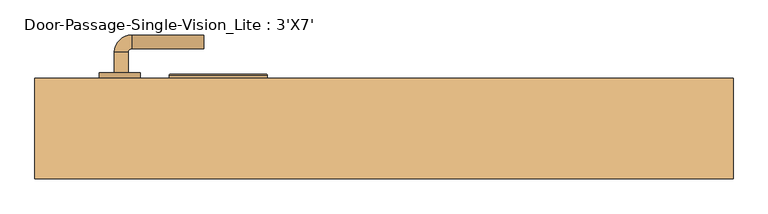
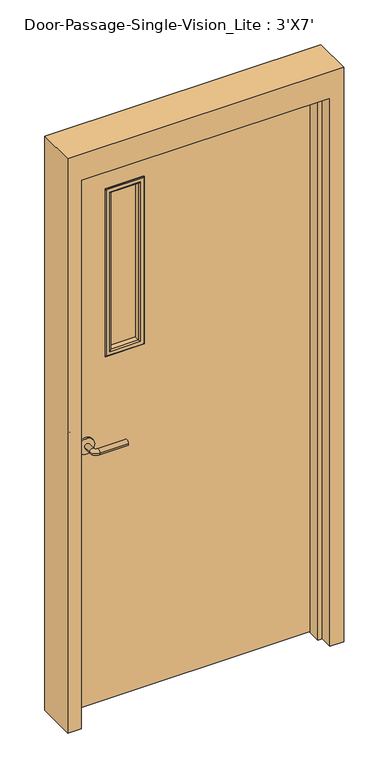
"""IFC4 building model written with IfcOpenShell, lengths in millimetres: door geometry, Door-Passage-Single-Vision_Lite : 3'X7'."""

from ifc_helpers import new_model, si_unit, point, frame, frame_2d, origin, place, context, project, spatial, polyline, circle_curve, ellipse_curve, trimmed, segment, composite_curve, outline, extrude, faceted_brep, source, transform, mapped, element, save
from ifc_brep_helpers import plane_surface, cylinder_surface, revolved_surface, advanced_brep


def door_passage_single_vision_lite_3_x7_440dd290(model_context):
    return source(origin(), model_context, "Body", "SolidModel", [
        advanced_brep(
        [(-392.190625, -14.35, 1016.0), (-372.190625, -14.35, 1016.0), (-372.190625, -44.35, 1016.0), (-392.190625, -44.35, 1016.0), (-367.190625, -49.35, 1016.0), (-367.190625, -69.35, 1016.0), (-262.190625, -69.35, 1016.0), (-262.190625, -49.35, 1016.0)],
        [
            (0, 1, circle_curve(frame((-382.190625, -14.35, 1016.0), z_axis=(0.0, 1.0, 0.0), x_axis=(1.0, 0.0, 0.0)), 10.0)),
            (1, 0, circle_curve(frame((-382.190625, -14.35, 1016.0), z_axis=(0.0, 1.0, 0.0), x_axis=(1.0, 0.0, 0.0)), 10.0)),
            (1, 2),
            (2, 3, circle_curve(frame((-382.190625, -44.35, 1016.0), z_axis=(0.0, 1.0, 0.0), x_axis=(1.0, 0.0, 0.0)), 10.0)),
            (3, 0),
            (3, 2, circle_curve(frame((-382.190625, -44.35, 1016.0), z_axis=(0.0, 1.0, 0.0), x_axis=(1.0, 0.0, 0.0)), 10.0)),
            (4, 5, circle_curve(frame((-367.190625, -59.35, 1016.0), z_axis=(-1.0, 0.0, 0.0), x_axis=(0.0, 1.0, 0.0)), 10.0)),
            (5, 3, circle_curve(frame((-367.190625, -44.35, 1016.0), z_axis=(0.0, 0.0, -1.0), x_axis=(-1.0, 0.0, 0.0)), 25.0)),
            (2, 4, circle_curve(frame((-367.190625, -44.35, 1016.0), z_axis=(0.0, 0.0, 1.0), x_axis=(-1.0, 0.0, 0.0)), 5.0)),
            (5, 4, circle_curve(frame((-367.190625, -59.35, 1016.0), z_axis=(-1.0, 0.0, 0.0), x_axis=(0.0, 1.0, 0.0)), 10.0)),
            (6, 7, circle_curve(frame((-262.190625, -59.35, 1016.0), z_axis=(1.0, 0.0, 0.0), x_axis=(0.0, 1.0, 0.0)), 10.0)),
            (7, 6, circle_curve(frame((-262.190625, -59.35, 1016.0), z_axis=(1.0, 0.0, 0.0), x_axis=(0.0, 1.0, 0.0)), 10.0)),
            (4, 7),
            (6, 5),
        ],
        [
            plane_surface(frame((-382.190625, -14.35, 1016.0), z_axis=(0.0, 1.0, 0.0), x_axis=(0.0, 0.0, 1.0))),
            cylinder_surface(frame((-382.190625, -14.35, 1016.0), z_axis=(0.0, 1.0, 0.0), x_axis=(1.0, 0.0, 0.0)), 10.0),
            revolved_surface(trimmed(ellipse_curve(frame((-382.190625, -44.35, 1016.0), z_axis=(0.0, -1.0, 0.0), x_axis=(1.0, 0.0, 0.0)), 10.0, 10.0), [point((-392.190625, -44.35, 1016.0))], [point((-372.190625, -44.35, 1016.0))], True, "CARTESIAN"), (-367.190625, -44.35, 1016.0), (0.0, 0.0, -1.0)),
            revolved_surface(trimmed(ellipse_curve(frame((-382.190625, -44.35, 1016.0), z_axis=(0.0, -1.0, 0.0), x_axis=(1.0, 0.0, 0.0)), 10.0, 10.0), [point((-372.190625, -44.35, 1016.0))], [point((-392.190625, -44.35, 1016.0))], True, "CARTESIAN"), (-367.190625, -44.35, 1016.0), (0.0, 0.0, -1.0)),
            plane_surface(frame((-262.190625, -59.35, 1016.0), z_axis=(1.0, 0.0, 0.0), x_axis=(0.0, 0.0, 1.0))),
            cylinder_surface(frame((-367.190625, -59.35, 1016.0), z_axis=(-1.0, 0.0, 0.0), x_axis=(0.0, 1.0, 0.0)), 10.0),
        ],
        [
            (0, [[1, 2]]),
            (1, [[3, 4, 5, -2]]),
            (1, [[-5, 6, -3, -1]]),
            (2, [[7, 8, -4, 9]]),
            (3, [[10, -9, -6, -8]]),
            (4, [[11, 12]]),
            (5, [[13, -11, 14, -7]]),
            (5, [[-14, -12, -13, -10]]),
        ],
    ),
        extrude(outline(composite_curve([segment(trimmed(circle_curve(frame_2d((1016.0, -384.690625)), 30.0), [point((1016.0, -414.690625))], [point((1016.0, -354.690625))], False, "CARTESIAN"), True, "CONTINUOUS"), segment(trimmed(circle_curve(frame_2d((1016.0, -384.690625)), 30.0), [point((1016.0, -354.690625))], [point((1016.0, -414.690625))], False, "CARTESIAN"), True, "CONTINUOUS")], self_intersect=False)), frame((0.0, -14.35, 0.0), z_axis=(0.0, 1.0, 0.0), x_axis=(0.0, 0.0, 1.0)), (0.0, 0.0, 1.0), 8.0),
        advanced_brep(
        [(-392.190625, 46.1, 1016.0), (-372.190625, 46.1, 1016.0), (-392.190625, 76.1, 1016.0), (-372.190625, 76.1, 1016.0), (-367.190625, 81.1, 1016.0), (-367.190625, 101.1, 1016.0), (-262.190625, 101.1, 1016.0), (-262.190625, 81.1, 1016.0)],
        [
            (0, 1, circle_curve(frame((-382.190625, 46.1, 1016.0), z_axis=(0.0, -1.0, 0.0), x_axis=(1.0, 0.0, 0.0)), 10.0)),
            (1, 0, circle_curve(frame((-382.190625, 46.1, 1016.0), z_axis=(0.0, -1.0, 0.0), x_axis=(1.0, 0.0, 0.0)), 10.0)),
            (0, 2),
            (2, 3, circle_curve(frame((-382.190625, 76.1, 1016.0), z_axis=(0.0, -1.0, 0.0), x_axis=(1.0, 0.0, 0.0)), 10.0)),
            (3, 1),
            (3, 2, circle_curve(frame((-382.190625, 76.1, 1016.0), z_axis=(0.0, -1.0, 0.0), x_axis=(1.0, 0.0, 0.0)), 10.0)),
            (4, 3, circle_curve(frame((-367.190625, 76.1, 1016.0), z_axis=(0.0, 0.0, 1.0), x_axis=(-1.0, 0.0, 0.0)), 5.0)),
            (2, 5, circle_curve(frame((-367.190625, 76.1, 1016.0), z_axis=(0.0, 0.0, -1.0), x_axis=(-1.0, 0.0, 0.0)), 25.0)),
            (5, 4, circle_curve(frame((-367.190625, 91.1, 1016.0), z_axis=(-1.0, 0.0, 0.0), x_axis=(0.0, -1.0, 0.0)), 10.0)),
            (4, 5, circle_curve(frame((-367.190625, 91.1, 1016.0), z_axis=(-1.0, 0.0, 0.0), x_axis=(0.0, -1.0, 0.0)), 10.0)),
            (6, 7, circle_curve(frame((-262.190625, 91.1, 1016.0), z_axis=(1.0, 0.0, 0.0), x_axis=(0.0, -1.0, 0.0)), 10.0)),
            (7, 6, circle_curve(frame((-262.190625, 91.1, 1016.0), z_axis=(1.0, 0.0, 0.0), x_axis=(0.0, -1.0, 0.0)), 10.0)),
            (5, 6),
            (7, 4),
        ],
        [
            plane_surface(frame((-382.190625, 46.1, 1016.0), z_axis=(0.0, -1.0, 0.0), x_axis=(0.0, 0.0, 1.0))),
            cylinder_surface(frame((-382.190625, 46.1, 1016.0), z_axis=(0.0, -1.0, 0.0), x_axis=(1.0, 0.0, 0.0)), 10.0),
            revolved_surface(trimmed(ellipse_curve(frame((-382.190625, 76.1, 1016.0), z_axis=(0.0, -1.0, 0.0), x_axis=(1.0, 0.0, 0.0)), 10.0, 10.0), [point((-392.190625, 76.1, 1016.0))], [point((-372.190625, 76.1, 1016.0))], True, "CARTESIAN"), (-367.190625, 76.1, 1016.0), (0.0, 0.0, -1.0)),
            revolved_surface(trimmed(ellipse_curve(frame((-382.190625, 76.1, 1016.0), z_axis=(0.0, -1.0, 0.0), x_axis=(1.0, 0.0, 0.0)), 10.0, 10.0), [point((-372.190625, 76.1, 1016.0))], [point((-392.190625, 76.1, 1016.0))], True, "CARTESIAN"), (-367.190625, 76.1, 1016.0), (0.0, 0.0, -1.0)),
            plane_surface(frame((-262.190625, 91.1, 1016.0), z_axis=(1.0, 0.0, 0.0), x_axis=(0.0, 0.0, 1.0))),
            cylinder_surface(frame((-367.190625, 91.1, 1016.0), z_axis=(-1.0, 0.0, 0.0), x_axis=(0.0, -1.0, 0.0)), 10.0),
        ],
        [
            (0, [[1, 2]]),
            (1, [[-1, 3, 4, 5]]),
            (1, [[-2, -5, 6, -3]]),
            (2, [[7, -4, 8, 9]]),
            (3, [[-8, -6, -7, 10]]),
            (4, [[11, 12]]),
            (5, [[-9, 13, -12, 14]]),
            (5, [[-10, -14, -11, -13]]),
        ],
    ),
        extrude(outline(composite_curve([segment(trimmed(circle_curve(frame_2d((1016.0, -384.690625)), 30.0), [point((1016.0, -414.690625))], [point((1016.0, -354.690625))], False, "CARTESIAN"), True, "CONTINUOUS"), segment(trimmed(circle_curve(frame_2d((1016.0, -384.690625)), 30.0), [point((1016.0, -354.690625))], [point((1016.0, -414.690625))], False, "CARTESIAN"), True, "CONTINUOUS")], self_intersect=False)), frame((0.0, 38.1, 0.0), z_axis=(0.0, 1.0, 0.0), x_axis=(0.0, 0.0, 1.0)), (0.0, 0.0, 1.0), 8.0),
        extrude(outline(polyline([(2133.6, -457.2), (0.0, -457.2), (0.0, 457.2), (2133.6, 457.2), (2133.6, -457.2)]), holes=[polyline([(1981.2, -304.8), (1981.2, -177.8), (1346.2, -177.8), (1346.2, -304.8), (1981.2, -304.8)])]), frame((0.0, -6.35, 0.0), z_axis=(0.0, 1.0, 0.0), x_axis=(0.0, 0.0, 1.0)), (0.0, 0.0, 1.0), 44.45),
        faceted_brep([(457.2, -11.1125, 0.0), (457.2, 38.1, 0.0), (508.0, 38.1, 0.0), (508.0, -107.95, 0.0), (457.2, -107.95, 0.0), (457.2, -58.7375, 0.0), (441.325, -58.7375, 0.0), (441.325, -11.1125, 0.0), (457.2, -11.1125, 2133.6), (457.2, 38.1, 2133.6), (-457.2, 38.1, 2133.6), (-457.2, 38.1, 0.0), (-508.0, 38.1, 0.0), (-508.0, 38.1, 2235.2), (508.0, 38.1, 2235.2), (508.0, -107.95, 2235.2), (-508.0, -107.95, 2235.2), (-508.0, -107.95, 0.0), (-457.2, -107.95, 0.0), (-457.2, -107.95, 2133.6), (457.2, -107.95, 2133.6), (457.2, -58.7375, 2133.6), (-457.2, -58.7375, 2133.6), (-457.2, -58.7375, 0.0), (-441.325, -58.7375, 0.0), (-441.325, -58.7375, 2117.725), (441.325, -58.7375, 2117.725), (441.325, -11.1125, 2117.725), (-441.325, -11.1125, 2117.725), (-441.325, -11.1125, 0.0), (-457.2, -11.1125, 0.0), (-457.2, -11.1125, 2133.6)], [[[0, 1, 2, 3, 4, 5, 6, 7]], [[1, 0, 8, 9]], [[2, 1, 9, 10, 11, 12, 13, 14]], [[3, 2, 14, 15]], [[4, 3, 15, 16, 17, 18, 19, 20]], [[5, 4, 20, 21]], [[6, 5, 21, 22, 23, 24, 25, 26]], [[7, 6, 26, 27]], [[0, 7, 27, 28, 29, 30, 31, 8]], [[9, 8, 31, 10]], [[20, 19, 22, 21]], [[26, 25, 28, 27]], [[12, 11, 30, 29, 24, 23, 18, 17]], [[11, 10, 31, 30]], [[13, 12, 17, 16]], [[19, 18, 23, 22]], [[25, 24, 29, 28]], [[15, 14, 13, 16]]]),
        extrude(outline(polyline([(-177.8, 12.7), (-304.8, 12.7), (-304.8, 19.05), (-177.8, 19.05), (-177.8, 12.7)])), frame((0.0, 0.0, 1346.2), z_axis=(0.0, 0.0, 1.0), x_axis=(1.0, 0.0, 0.0)), (0.0, 0.0, 1.0), 635.0),
        advanced_brep(
        [(-304.8, 19.05, 1981.2), (-304.8, 38.1, 1981.2), (-304.8, 38.1, 1346.2), (-304.8, 19.05, 1346.2), (-292.8, 39.1, 1969.2), (-292.8, 19.05, 1969.2), (-292.8, 19.05, 1358.2), (-292.8, 39.1, 1358.2), (-297.8, 44.1, 1974.2), (-297.8, 44.1, 1353.2), (-312.8, 42.1, 1989.2), (-310.8, 44.1, 1987.2), (-310.8, 44.1, 1340.2), (-312.8, 42.1, 1338.2), (-312.8, 38.1, 1989.2), (-312.8, 38.1, 1338.2), (-177.8, 38.1, 1346.2), (-177.8, 19.05, 1346.2), (-189.8, 19.05, 1358.2), (-189.8, 39.1, 1358.2), (-184.8, 44.1, 1353.2), (-171.8, 44.1, 1340.2), (-169.8, 42.1, 1338.2), (-169.8, 38.1, 1338.2), (-177.8, 38.1, 1981.2), (-177.8, 19.05, 1981.2), (-189.8, 19.05, 1969.2), (-189.8, 39.1, 1969.2), (-184.8, 44.1, 1974.2), (-171.8, 44.1, 1987.2), (-169.8, 42.1, 1989.2), (-169.8, 38.1, 1989.2)],
        [
            (0, 1),
            (1, 2),
            (2, 3),
            (3, 0),
            (4, 5),
            (5, 6),
            (6, 7),
            (7, 4),
            (8, 4, ellipse_curve(frame((-297.8, 39.1, 1974.2), z_axis=(-0.7071067811865475, 0.0, -0.7071067811865475), x_axis=(-0.7071067811865474, 0.0, 0.7071067811865476)), 7.0710678, 5.0)),
            (7, 9, ellipse_curve(frame((-297.8, 39.1, 1353.2), z_axis=(-0.7071067811865475, 0.0, 0.7071067811865475), x_axis=(0.7071067811865474, 0.0, 0.7071067811865476)), 7.0710678, 5.0)),
            (9, 8),
            (10, 11, ellipse_curve(frame((-310.8, 42.1, 1987.2), z_axis=(-0.7071067811865475, 0.0, -0.7071067811865475), x_axis=(-0.7071067811865474, 0.0, 0.7071067811865476)), 2.8284271, 2.0)),
            (11, 12),
            (12, 13, ellipse_curve(frame((-310.8, 42.1, 1340.2), z_axis=(-0.7071067811865475, 0.0, 0.7071067811865475), x_axis=(0.7071067811865474, 0.0, 0.7071067811865476)), 2.8284271, 2.0)),
            (13, 10),
            (14, 10),
            (13, 15),
            (15, 14),
            (2, 16),
            (16, 17),
            (17, 3),
            (6, 18),
            (18, 19),
            (19, 7),
            (19, 20, ellipse_curve(frame((-184.8, 39.1, 1353.2), z_axis=(-0.7071067811865475, 0.0, -0.7071067811865475), x_axis=(-0.7071067811865476, 0.0, 0.7071067811865474)), 7.0710678, 5.0)),
            (20, 9),
            (12, 21),
            (21, 22, ellipse_curve(frame((-171.8, 42.1, 1340.2), z_axis=(-0.7071067811865475, 0.0, -0.7071067811865475), x_axis=(-0.7071067811865476, 0.0, 0.7071067811865474)), 2.8284271, 2.0)),
            (22, 13),
            (22, 23),
            (23, 15),
            (16, 24),
            (24, 25),
            (25, 17),
            (18, 26),
            (26, 27),
            (27, 19),
            (27, 28, ellipse_curve(frame((-184.8, 39.1, 1974.2), z_axis=(0.7071067811865475, 0.0, -0.7071067811865475), x_axis=(-0.7071067811865474, 0.0, -0.7071067811865476)), 7.0710678, 5.0)),
            (28, 20),
            (21, 29),
            (29, 30, ellipse_curve(frame((-171.8, 42.1, 1987.2), z_axis=(0.7071067811865475, 0.0, -0.7071067811865475), x_axis=(-0.7071067811865474, 0.0, -0.7071067811865476)), 2.8284271, 2.0)),
            (30, 22),
            (30, 31),
            (31, 23),
            (31, 14),
            (1, 24),
            (0, 25),
            (5, 26),
            (4, 27),
            (8, 28),
            (11, 29),
            (10, 30),
        ],
        [
            plane_surface(frame((-304.8, 38.1, 1981.2), z_axis=(-1.0, 0.0, 0.0), x_axis=(0.0, 0.0, -1.0))),
            plane_surface(frame((-292.8, 19.05, 1969.2), z_axis=(1.0, 0.0, 0.0), x_axis=(0.0, 0.0, -1.0))),
            cylinder_surface(frame((-297.8, 39.1, 1981.2), z_axis=(0.0, 0.0, 1.0), x_axis=(-1.0, 0.0, 0.0)), 5.0),
            cylinder_surface(frame((-310.8, 42.1, 1981.2), z_axis=(0.0, 0.0, 1.0), x_axis=(-1.0, 0.0, 0.0)), 2.0),
            plane_surface(frame((-312.8, 42.1, 1989.2), z_axis=(-1.0, 0.0, 0.0), x_axis=(0.0, 0.0, -1.0))),
            plane_surface(frame((-304.8, 38.1, 1346.2), z_axis=(0.0, 0.0, -1.0), x_axis=(1.0, 0.0, 0.0))),
            plane_surface(frame((-292.8, 19.05, 1358.2), z_axis=(0.0, 0.0, 1.0), x_axis=(1.0, 0.0, 0.0))),
            cylinder_surface(frame((-304.8, 39.1, 1353.2), z_axis=(-1.0, 0.0, 0.0), x_axis=(0.0, 0.0, -1.0)), 5.0),
            cylinder_surface(frame((-304.8, 42.1, 1340.2), z_axis=(-1.0, 0.0, 0.0), x_axis=(0.0, 0.0, -1.0)), 2.0),
            plane_surface(frame((-312.8, 42.1, 1338.2), z_axis=(0.0, 0.0, -1.0), x_axis=(1.0, 0.0, 0.0))),
            plane_surface(frame((-177.8, 38.1, 1346.2), z_axis=(1.0, 0.0, 0.0), x_axis=(0.0, 0.0, 1.0))),
            plane_surface(frame((-189.8, 19.05, 1358.2), z_axis=(-1.0, 0.0, 0.0), x_axis=(0.0, 0.0, 1.0))),
            cylinder_surface(frame((-184.8, 39.1, 1346.2), z_axis=(0.0, 0.0, -1.0), x_axis=(1.0, 0.0, 0.0)), 5.0),
            cylinder_surface(frame((-171.8, 42.1, 1346.2), z_axis=(0.0, 0.0, -1.0), x_axis=(1.0, 0.0, 0.0)), 2.0),
            plane_surface(frame((-169.8, 42.1, 1338.2), z_axis=(1.0, 0.0, 0.0), x_axis=(0.0, 0.0, 1.0))),
            plane_surface(frame((-169.8, 38.1, 1989.2), z_axis=(0.0, -1.0, 0.0), x_axis=(-1.0, 0.0, 0.0))),
            plane_surface(frame((-177.8, 38.1, 1981.2), z_axis=(0.0, 0.0, 1.0), x_axis=(-1.0, 0.0, 0.0))),
            plane_surface(frame((-177.8, 19.05, 1981.2), z_axis=(0.0, -1.0, 0.0), x_axis=(-1.0, 0.0, 0.0))),
            plane_surface(frame((-189.8, 19.05, 1969.2), z_axis=(0.0, 0.0, -1.0), x_axis=(-1.0, 0.0, 0.0))),
            cylinder_surface(frame((-177.8, 39.1, 1974.2), z_axis=(1.0, 0.0, 0.0), x_axis=(0.0, 0.0, 1.0)), 5.0),
            plane_surface(frame((-184.8, 44.1, 1974.2), z_axis=(0.0, 1.0, 0.0), x_axis=(-1.0, 0.0, 0.0))),
            cylinder_surface(frame((-177.8, 42.1, 1987.2), z_axis=(1.0, 0.0, 0.0), x_axis=(0.0, 0.0, 1.0)), 2.0),
            plane_surface(frame((-169.8, 42.1, 1989.2), z_axis=(0.0, 0.0, 1.0), x_axis=(-1.0, 0.0, 0.0))),
        ],
        [
            (0, [[1, 2, 3, 4]]),
            (1, [[5, 6, 7, 8]]),
            (2, [[9, -8, 10, 11]]),
            (3, [[12, 13, 14, 15]]),
            (4, [[16, -15, 17, 18]]),
            (5, [[-3, 19, 20, 21]]),
            (6, [[-7, 22, 23, 24]]),
            (7, [[-10, -24, 25, 26]]),
            (8, [[-14, 27, 28, 29]]),
            (9, [[-17, -29, 30, 31]]),
            (10, [[-20, 32, 33, 34]]),
            (11, [[-23, 35, 36, 37]]),
            (12, [[-25, -37, 38, 39]]),
            (13, [[-28, 40, 41, 42]]),
            (14, [[-30, -42, 43, 44]]),
            (15, [[-31, -44, 45, -18], [46, -32, -19, -2]]),
            (16, [[-33, -46, -1, 47]]),
            (17, [[-21, -34, -47, -4], [48, -35, -22, -6]]),
            (18, [[-36, -48, -5, 49]]),
            (19, [[-38, -49, -9, 50]]),
            (20, [[51, -40, -27, -13], [-26, -39, -50, -11]]),
            (21, [[-41, -51, -12, 52]]),
            (22, [[-43, -52, -16, -45]]),
        ],
    ),
        advanced_brep(
        [(-304.8, 12.7, 1346.2), (-304.8, -6.35, 1346.2), (-304.8, -6.35, 1981.2), (-304.8, 12.7, 1981.2), (-292.8, -7.35, 1358.2), (-292.8, 12.7, 1358.2), (-292.8, 12.7, 1969.2), (-292.8, -7.35, 1969.2), (-297.8, -12.35, 1353.2), (-297.8, -12.35, 1974.2), (-312.8, -10.35, 1338.2), (-310.8, -12.35, 1340.2), (-310.8, -12.35, 1987.2), (-312.8, -10.35, 1989.2), (-312.8, -6.35, 1338.2), (-312.8, -6.35, 1989.2), (-177.8, -6.35, 1981.2), (-177.8, 12.7, 1981.2), (-189.8, 12.7, 1969.2), (-189.8, -7.35, 1969.2), (-184.8, -12.35, 1974.2), (-171.8, -12.35, 1987.2), (-169.8, -10.35, 1989.2), (-169.8, -6.35, 1989.2), (-177.8, -6.35, 1346.2), (-177.8, 12.7, 1346.2), (-189.8, 12.7, 1358.2), (-189.8, -7.35, 1358.2), (-184.8, -12.35, 1353.2), (-171.8, -12.35, 1340.2), (-169.8, -10.35, 1338.2), (-169.8, -6.35, 1338.2)],
        [
            (0, 1),
            (1, 2),
            (2, 3),
            (3, 0),
            (4, 5),
            (5, 6),
            (6, 7),
            (7, 4),
            (8, 4, ellipse_curve(frame((-297.8, -7.35, 1353.2), z_axis=(-0.7071067811865475, 0.0, 0.7071067811865475), x_axis=(-0.7071067811865474, 0.0, -0.7071067811865476)), 7.0710678, 5.0)),
            (7, 9, ellipse_curve(frame((-297.8, -7.35, 1974.2), z_axis=(-0.7071067811865475, 0.0, -0.7071067811865475), x_axis=(0.7071067811865474, 0.0, -0.7071067811865476)), 7.0710678, 5.0)),
            (9, 8),
            (10, 11, ellipse_curve(frame((-310.8, -10.35, 1340.2), z_axis=(-0.7071067811865475, 0.0, 0.7071067811865475), x_axis=(-0.7071067811865474, 0.0, -0.7071067811865476)), 2.8284271, 2.0)),
            (11, 12),
            (12, 13, ellipse_curve(frame((-310.8, -10.35, 1987.2), z_axis=(-0.7071067811865475, 0.0, -0.7071067811865475), x_axis=(0.7071067811865474, 0.0, -0.7071067811865476)), 2.8284271, 2.0)),
            (13, 10),
            (14, 10),
            (13, 15),
            (15, 14),
            (2, 16),
            (16, 17),
            (17, 3),
            (6, 18),
            (18, 19),
            (19, 7),
            (19, 20, ellipse_curve(frame((-184.8, -7.35, 1974.2), z_axis=(-0.7071067811865475, 0.0, 0.7071067811865475), x_axis=(-0.7071067811865476, 0.0, -0.7071067811865474)), 7.0710678, 5.0)),
            (20, 9),
            (12, 21),
            (21, 22, ellipse_curve(frame((-171.8, -10.35, 1987.2), z_axis=(-0.7071067811865475, 0.0, 0.7071067811865475), x_axis=(-0.7071067811865476, 0.0, -0.7071067811865474)), 2.8284271, 2.0)),
            (22, 13),
            (22, 23),
            (23, 15),
            (16, 24),
            (24, 25),
            (25, 17),
            (18, 26),
            (26, 27),
            (27, 19),
            (27, 28, ellipse_curve(frame((-184.8, -7.35, 1353.2), z_axis=(0.7071067811865475, 0.0, 0.7071067811865475), x_axis=(-0.7071067811865474, 0.0, 0.7071067811865476)), 7.0710678, 5.0)),
            (28, 20),
            (21, 29),
            (29, 30, ellipse_curve(frame((-171.8, -10.35, 1340.2), z_axis=(0.7071067811865475, 0.0, 0.7071067811865475), x_axis=(-0.7071067811865474, 0.0, 0.7071067811865476)), 2.8284271, 2.0)),
            (30, 22),
            (30, 31),
            (31, 23),
            (31, 14),
            (1, 24),
            (0, 25),
            (5, 26),
            (4, 27),
            (8, 28),
            (11, 29),
            (10, 30),
        ],
        [
            plane_surface(frame((-304.8, -6.35, 1346.2), z_axis=(-1.0, 0.0, 0.0), x_axis=(0.0, 0.0, 1.0))),
            plane_surface(frame((-292.8, 12.7, 1358.2), z_axis=(1.0, 0.0, 0.0), x_axis=(0.0, 0.0, 1.0))),
            cylinder_surface(frame((-297.8, -7.35, 1346.2), z_axis=(0.0, 0.0, -1.0), x_axis=(-1.0, 0.0, 0.0)), 5.0),
            cylinder_surface(frame((-310.8, -10.35, 1346.2), z_axis=(0.0, 0.0, -1.0), x_axis=(-1.0, 0.0, 0.0)), 2.0),
            plane_surface(frame((-312.8, -10.35, 1338.2), z_axis=(-1.0, 0.0, 0.0), x_axis=(0.0, 0.0, 1.0))),
            plane_surface(frame((-304.8, -6.35, 1981.2), z_axis=(0.0, 0.0, 1.0), x_axis=(1.0, 0.0, 0.0))),
            plane_surface(frame((-292.8, 12.7, 1969.2), z_axis=(0.0, 0.0, -1.0), x_axis=(1.0, 0.0, 0.0))),
            cylinder_surface(frame((-304.8, -7.35, 1974.2), z_axis=(-1.0, 0.0, 0.0), x_axis=(0.0, 0.0, 1.0)), 5.0),
            cylinder_surface(frame((-304.8, -10.35, 1987.2), z_axis=(-1.0, 0.0, 0.0), x_axis=(0.0, 0.0, 1.0)), 2.0),
            plane_surface(frame((-312.8, -10.35, 1989.2), z_axis=(0.0, 0.0, 1.0), x_axis=(1.0, 0.0, 0.0))),
            plane_surface(frame((-177.8, -6.35, 1981.2), z_axis=(1.0, 0.0, 0.0), x_axis=(0.0, 0.0, -1.0))),
            plane_surface(frame((-189.8, 12.7, 1969.2), z_axis=(-1.0, 0.0, 0.0), x_axis=(0.0, 0.0, -1.0))),
            cylinder_surface(frame((-184.8, -7.35, 1981.2), z_axis=(0.0, 0.0, 1.0), x_axis=(1.0, 0.0, 0.0)), 5.0),
            cylinder_surface(frame((-171.8, -10.35, 1981.2), z_axis=(0.0, 0.0, 1.0), x_axis=(1.0, 0.0, 0.0)), 2.0),
            plane_surface(frame((-169.8, -10.35, 1989.2), z_axis=(1.0, 0.0, 0.0), x_axis=(0.0, 0.0, -1.0))),
            plane_surface(frame((-169.8, -6.35, 1338.2), z_axis=(0.0, 1.0, 0.0), x_axis=(-1.0, 0.0, 0.0))),
            plane_surface(frame((-177.8, -6.35, 1346.2), z_axis=(0.0, 0.0, -1.0), x_axis=(-1.0, 0.0, 0.0))),
            plane_surface(frame((-177.8, 12.7, 1346.2), z_axis=(0.0, 1.0, 0.0), x_axis=(-1.0, 0.0, 0.0))),
            plane_surface(frame((-189.8, 12.7, 1358.2), z_axis=(0.0, 0.0, 1.0), x_axis=(-1.0, 0.0, 0.0))),
            cylinder_surface(frame((-177.8, -7.35, 1353.2), z_axis=(1.0, 0.0, 0.0), x_axis=(0.0, 0.0, -1.0)), 5.0),
            plane_surface(frame((-184.8, -12.35, 1353.2), z_axis=(0.0, -1.0, 0.0), x_axis=(-1.0, 0.0, 0.0))),
            cylinder_surface(frame((-177.8, -10.35, 1340.2), z_axis=(1.0, 0.0, 0.0), x_axis=(0.0, 0.0, -1.0)), 2.0),
            plane_surface(frame((-169.8, -10.35, 1338.2), z_axis=(0.0, 0.0, -1.0), x_axis=(-1.0, 0.0, 0.0))),
        ],
        [
            (0, [[1, 2, 3, 4]]),
            (1, [[5, 6, 7, 8]]),
            (2, [[9, -8, 10, 11]]),
            (3, [[12, 13, 14, 15]]),
            (4, [[16, -15, 17, 18]]),
            (5, [[-3, 19, 20, 21]]),
            (6, [[-7, 22, 23, 24]]),
            (7, [[-10, -24, 25, 26]]),
            (8, [[-14, 27, 28, 29]]),
            (9, [[-17, -29, 30, 31]]),
            (10, [[-20, 32, 33, 34]]),
            (11, [[-23, 35, 36, 37]]),
            (12, [[-25, -37, 38, 39]]),
            (13, [[-28, 40, 41, 42]]),
            (14, [[-30, -42, 43, 44]]),
            (15, [[-31, -44, 45, -18], [46, -32, -19, -2]]),
            (16, [[-33, -46, -1, 47]]),
            (17, [[-21, -34, -47, -4], [48, -35, -22, -6]]),
            (18, [[-36, -48, -5, 49]]),
            (19, [[-38, -49, -9, 50]]),
            (20, [[51, -40, -27, -13], [-26, -39, -50, -11]]),
            (21, [[-41, -51, -12, 52]]),
            (22, [[-43, -52, -16, -45]]),
        ],
    ),
    ])


if __name__ == "__main__":
    model = new_model("IFC4")
    model_context = context("Model", 3, world=origin())
    ifc_project = project(units=[si_unit("LENGTHUNIT", "METRE", prefix="MILLI")], contexts=[model_context])
    site = spatial("IfcSite", under=ifc_project)
    building = spatial("IfcBuilding", under=site)
    placement = place(None, origin())
    door_passage_single_vision_lite_3_x7_shape = door_passage_single_vision_lite_3_x7_440dd290(model_context)
    element("IfcDoor", 1, ObjectType="Door-Passage-Single-Vision_Lite : 3'X7'", at=placement, inside=building, context=model_context, shape_type="MappedRepresentation", body=[
        mapped(door_passage_single_vision_lite_3_x7_shape, transform((0.0, 0.0, 0.0), x_axis=(1.0, 0.0, 0.0), y_axis=(0.0, 1.0, 0.0), z_axis=(0.0, 0.0, 1.0))),
    ])
    save(model, "model.ifc")

# Revit data of these elements
# Type "Door-Passage-Single-Vision_Lite : 3'X7'"
#   Type Mark = "9"
#   Assembly Code = "B2030100"
#   Analytic Construction = "Wooden"
#   Thickness = 0' - 1 3/4"
#   Thermal Resistance (R) = 2.5876 (h·ft²·°F)/BTU
#   Swing Angle [instance default] = 90.00°
#   Strike Height = 3' - 4"
#   Rough Width [instance default] = 3' - 4"
#   Rough Height [instance default] = 7' - 4"
#   MFOpeningHeight [instance default] = 0' - 4"
#   MFOpeningWidth [instance default] = 0' - 4"
#   Inset Calculate [instance default] = 0' - 4"
#   Masonry Inset [instance default] = 0' - 1"
#   Height = 7' - 0"
#   Width = 3' - 0"
#   Heat Transfer Coefficient (U) = 0.3865 BTU/(h·ft²·°F)
#   Masonry Frame Depth = 0' - 5 3/4"
#   Masonry Frame [instance default] = yes
#   Function = 1
#   Dry Wall Frame [instance default] = no
#   Panel Material = Wood - Birch
#   Glazing = Glass
#   Glass Stop Material = Metal - Paint Finish - Grey
#   Frame Material = Metal - Paint Finish - Grey
#   Door Handle Material = Aluminum
#   Visual Light Transmittance = 0
#   Solar Heat Gain Coefficient = 0
#   Wall Closure = (empty or 0)
# Element 1 (IfcDoor, "Door-Passage-Single-Vision_Lite : 3'X7'")
#   Materials on its faces: "Metal - Paint Finish - Grey", "Aluminum", "Wood - Birch", "Glass"
# Materials
#   "Wood - Birch": class "Wood", colour RGB 166 116 52, transparency 0, Cost = 0
#   "Glass": class "Glass", colour RGB 0 128 192, transparency 0.75, Description = "Soda Lime Glass", Cost = 0
#   "Metal - Paint Finish - Grey": class "Paint", colour RGB 104 104 104, transparency 0, Cost = 0
#   "Aluminum": class "Metal", colour RGB 247 247 247, transparency 0, Description = "Aluminum 6061", Cost = 0
